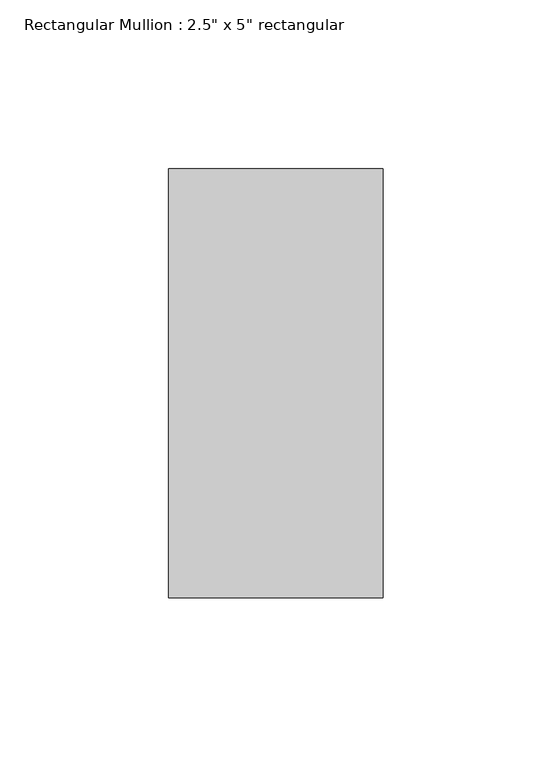
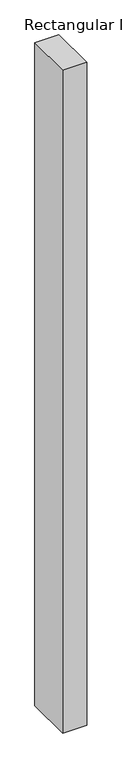
"""IFC4 building model written with IfcOpenShell, lengths in millimetres: member geometry."""

from ifc_helpers import new_model, si_unit, frame, origin, place, context, project, spatial, polyline, outline, extrude, source, transform, mapped, element, save


def member_bcae55ac(model_context):
    return source(origin(), model_context, "Body", "SweptSolid", [
        extrude(outline(polyline([(31.75, 63.5), (31.75, -63.5), (-31.75, -63.5), (-31.75, 63.5), (31.75, 63.5)])), frame((0.0, 0.0, -1852.7814546), z_axis=(0.0, 0.0, 1.0), x_axis=(1.0, 0.0, 0.0)), (0.0, 0.0, 1.0), 1852.7814546),
    ])


if __name__ == "__main__":
    model = new_model("IFC4")
    model_context = context("Model", 3, world=origin())
    ifc_project = project(units=[si_unit("LENGTHUNIT", "METRE", prefix="MILLI")], contexts=[model_context])
    site = spatial("IfcSite", under=ifc_project)
    building = spatial("IfcBuilding", under=site)
    placement = place(None, origin())
    member_shape = member_bcae55ac(model_context)
    element("IfcMember", 1, ObjectType="Rectangular Mullion : 2.5\" x 5\" rectangular", at=placement, inside=building, context=model_context, shape_type="MappedRepresentation", body=[
        mapped(member_shape, transform((0.0, 0.0, 0.0), x_axis=(1.0, 0.0, 0.0), y_axis=(0.0, 1.0, 0.0), z_axis=(0.0, 0.0, 1.0))),
    ])
    save(model, "model.ifc")

# Revit data of these elements
# Type "Rectangular Mullion : 2.5\" x 5\" rectangular"
#   built-in parameter 1007304 = 0.416667 (stored number, unit not read)
#   built-in parameter 1007301 = 0.104167 (stored number, unit not read)
#   built-in parameter 1007300 = 0.104167 (stored number, unit not read)
# Element 1 (IfcMember, "Rectangular Mullion : 2.5\" x 5\" rectangular")
#   Materials on its faces: "Aluminum"
# Materials
#   "Aluminum": class "Metal", colour RGB 247 247 247, transparency 0, Description = "Aluminum 6061", Cost = 0
